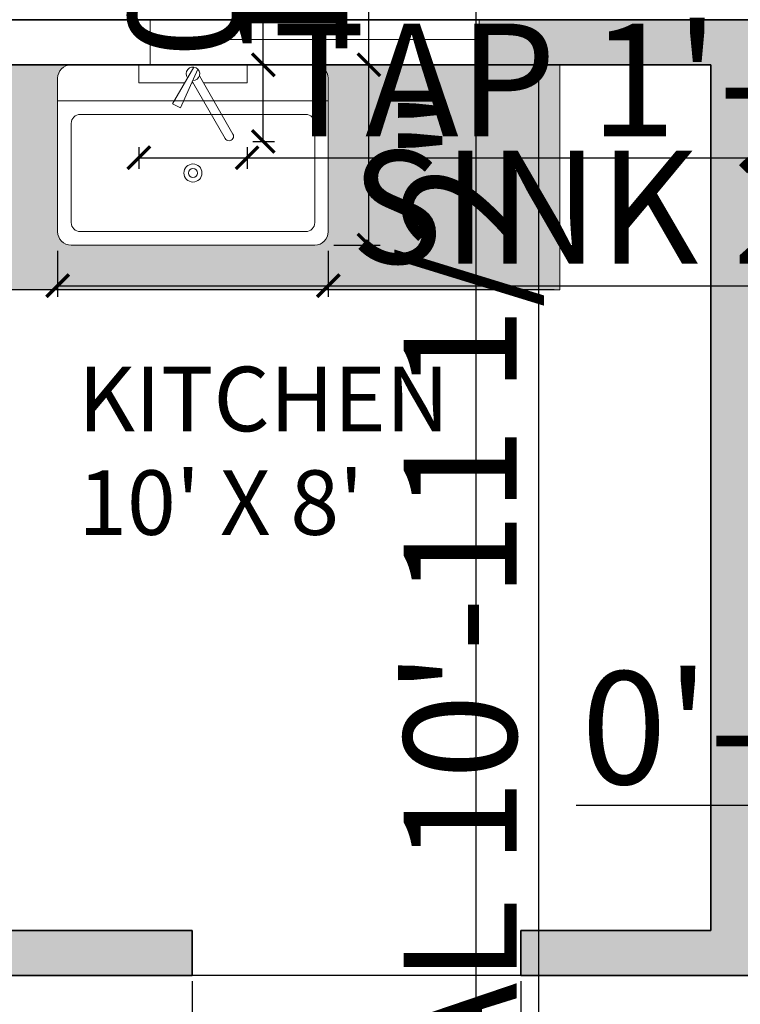
# Model space of a CAD drawing. Units: inches. Extents: x 1763 to 2368, y 1500 to 2097.
# Tile 8 of 24: x 1876 to 1956, y 1877 to 1986. Entities that reach past the tile are written whole.
import ezdxf

# ---------------------------------------------------------------- set-up
doc = ezdxf.new("R2010")
doc.units = ezdxf.units.IN
for name, color, linetype, lineweight in [('A-ANNO-DIMS', 2, 'Continuous', 18), ('A-AREA-IDEN', 7, 'Continuous', 18), ('A-FLOR-CASE', 8, 'Continuous', 18), ('A-FLOR-FIXT', 9, 'Continuous', 18), ('A-WALL', 7, 'Continuous', 35), ('A-WALL-PATT', 7, 'Continuous', 13), ('windows', 1, 'Continuous', 18)]:
    doc.layers.add(name, color=color, linetype=linetype, lineweight=lineweight)
doc.layers.add('A-FLOR-CASE-PATT', color=254, linetype='Continuous', lineweight=13, true_color=0xcecce6)
doc.styles.get("Standard").update_dxf_attribs({"font": 'arial.ttf'})
doc.dimstyles.new('ISO-25', dxfattribs={"dimtxt": 12.5, "dimasz": 2.5, "dimexe": 1.25, "dimexo": 0.625, "dimtad": 1, "dimdec": 0, "dimlunit": 4, "dimtxsty": 'Standard', "dimblk": 'ARCHTICK', "dimcen": 2.5, "dimclrd": 3, "dimclrt": 4, "dimadec": 0, "dimazin": 0, "dimtfac": 1, "dimtdec": 0, "dimtmove": 0, "dimatfit": 3, "dimfxl": 1, "dimarcsym": 0})

# ---------------------------------------------------------------- blocks, each defined once
blk = doc.blocks.new('Faucet - single handle top')
for p, q in [((0.08, -0.26), (-2.26, -4.34)), ((-1.37, -4.79), (0.55, -0.5)), ((-0.06, -1.9), (3.57, -8.18)), ((4.43, -7.68), (0.72, -1.24)), ((-2.26, -4.34), (-1.37, -4.79))]:
    blk.add_line(p, q)
for points in [[(-0.92, -2), (-6, -2), (-6, 0), (6, 0), (6, -2), (1.16, -2)], [(-0.01, -2), (-0.12, -2)]]:
    blk.add_lwpolyline(points)
for centre, radius, start, end in [((0, -1), 0.75, 269.2246, 216.2304), ((4, -7.93), 0.5, 210, 30)]:
    blk.add_arc(centre, radius, start, end)
blk = doc.blocks.new('Sink-single - 30 in top')
blk.add_line((-15, -3.999996), (15, -3.999996))
for points in [[(-13.5, 0), (13.5, 0)], [(-15, -18.499996), (-15, -1.5)], [(15, -1.5), (15, -18.499996)], [(-13.5, -17.499996), (-13.5, -6.499996)], [(-12.5, -5.499996), (12.5, -5.499996)], [(13.5, -6.499996), (13.5, -17.499996)], [(12.5, -18.499996), (-12.5, -18.499996)], [(13.5, -19.999996), (-13.5, -19.999996)]]:
    blk.add_lwpolyline(points)
for radius in [1, 0.5]:
    blk.add_circle((0, -11.999996), radius)
for centre, radius, start, end in [((-13.5, -1.5), 1.5, 90, 180), ((13.5, -1.5), 1.5, 0, 90), ((-12.5, -6.499996), 1, 90, 180), ((12.5, -6.499996), 1, 0, 90), ((-13.5, -18.499996), 1.5, 180, 270), ((-12.5, -17.499996), 1, 180, 270), ((12.5, -17.499996), 1, 270, 0), ((13.5, -18.499996), 1.5, 270, 0)]:
    blk.add_arc(centre, radius, start, end)
blk = doc.blocks.new('_ArchTick')
at = {"color": 0, "linetype": 'ByBlock', "const_width": 0.15}
blk.add_lwpolyline([(-0.5, -0.5), (0.5, 0.5)], dxfattribs=at)
blk = doc.blocks.new('*D25')
at = {"layer": 'A-ANNO-DIMS', "color": 3, "lineweight": -2, "transparency": 16777216}
for p, q in [((1934.01, 1792.31), (1934.01, 1981.61)), ((1934.01, 1660.94), (1934.01, 1792.31))]:
    blk.add_line(p, q, dxfattribs=at)
at = {"layer": 'A-ANNO-DIMS', "color": 0, "lineweight": -2, "transparency": 16777216}
for p, q in [((1953.09, 1792.31), (1932.76, 1792.31)), ((1953.09, 1660.94), (1932.76, 1660.94))]:
    blk.add_line(p, q, dxfattribs=at)
at = {"layer": 'Defpoints', "color": 0, "transparency": 16777216}
for p in [(1934.01, 1792.31), (1953.72, 1792.31), (1953.72, 1660.94)]:
    blk.add_point(p, dxfattribs=at)
at = {"layer": 'A-ANNO-DIMS', "color": 3, "lineweight": -2, "transparency": 16777216, "xscale": 2.5, "yscale": 2.5, "zscale": 2.5}
for p, rotation in [((1934.01, 1792.31), 90), ((1934.01, 1660.94), 270)]:
    blk.add_blockref('_ArchTick', p, dxfattribs=dict(at, rotation=rotation))
at = {"layer": 'A-ANNO-DIMS', "color": 4, "transparency": 16777216, "insert": (1926.92, 1888.21), "char_height": 12.5, "attachment_point": 5, "rotation": 90}
blk.add_mtext('SECTIONAL 10\'-11 1/2"', dxfattribs=at)
blk = doc.blocks.new('*D29')
at = {"layer": 'A-ANNO-DIMS', "color": 3, "lineweight": -2, "transparency": 16777216}
for p, q in [((1868.59, 1924.21), (1868.59, 2027.49)), ((1868.59, 1894.21), (1868.59, 1924.21))]:
    blk.add_line(p, q, dxfattribs=at)
at = {"layer": 'A-ANNO-DIMS', "color": 0, "lineweight": -2, "transparency": 16777216}
for p, q in [((1864.72, 1924.21), (1869.84, 1924.21)), ((1864.72, 1894.21), (1869.84, 1894.21))]:
    blk.add_line(p, q, dxfattribs=at)
at = {"layer": 'Defpoints', "color": 0, "transparency": 16777216}
for p in [(1864.09, 1924.21), (1868.59, 1924.21), (1864.09, 1894.21)]:
    blk.add_point(p, dxfattribs=at)
at = {"layer": 'A-ANNO-DIMS', "color": 3, "lineweight": -2, "transparency": 16777216, "xscale": 2.5, "yscale": 2.5, "zscale": 2.5}
for p, rotation in [((1868.59, 1924.21), 90), ((1868.59, 1894.21), 270)]:
    blk.add_blockref('_ArchTick', p, dxfattribs=dict(at, rotation=rotation))
at = {"layer": 'A-ANNO-DIMS', "color": 4, "transparency": 16777216, "insert": (1861.5, 1977.1), "char_height": 12.5, "attachment_point": 5, "rotation": 90}
blk.add_mtext('RANGE 2\'-6"', dxfattribs=at)
blk = doc.blocks.new('*D31')
at = {"layer": 'A-ANNO-DIMS', "color": 0, "lineweight": -2, "transparency": 16777216}
for p, q in [((1880.68, 1960.65), (1880.68, 1955.52)), ((1910.68, 1960.65), (1910.68, 1955.52))]:
    blk.add_line(p, q, dxfattribs=at)
at = {"layer": 'A-ANNO-DIMS', "color": 3, "lineweight": -2, "transparency": 16777216}
for p, q in [((1880.68, 1956.77), (1910.68, 1956.77)), ((1910.68, 1956.77), (1993.21, 1956.77))]:
    blk.add_line(p, q, dxfattribs=at)
at = {"layer": 'Defpoints', "color": 0, "transparency": 16777216}
for p in [(1880.68, 1961.27), (1910.68, 1961.27), (1910.68, 1956.77)]:
    blk.add_point(p, dxfattribs=at)
at = {"layer": 'A-ANNO-DIMS', "color": 3, "lineweight": -2, "transparency": 16777216, "xscale": 2.5, "yscale": 2.5, "zscale": 2.5, "rotation": 180}
blk.add_blockref('_ArchTick', (1880.68, 1956.77), dxfattribs=at)
at = {"layer": 'A-ANNO-DIMS', "color": 3, "lineweight": -2, "transparency": 16777216, "xscale": 2.5, "yscale": 2.5, "zscale": 2.5}
blk.add_blockref('_ArchTick', (1910.68, 1956.77), dxfattribs=at)
at = {"layer": 'A-ANNO-DIMS', "color": 4, "transparency": 16777216, "insert": (1953.2, 1963.86), "char_height": 12.5, "attachment_point": 5}
blk.add_mtext('SINK 2\'-6"', dxfattribs=at)
blk = doc.blocks.new('*D32')
at = {"layer": 'A-ANNO-DIMS', "color": 3, "lineweight": -2, "transparency": 16777216}
for p, q in [((1915.18, 1981.27), (1915.18, 2017.07)), ((1915.18, 1961.27), (1915.18, 1981.27))]:
    blk.add_line(p, q, dxfattribs=at)
at = {"layer": 'A-ANNO-DIMS', "color": 0, "lineweight": -2, "transparency": 16777216}
for p, q in [((1911.31, 1981.27), (1916.43, 1981.27)), ((1911.31, 1961.27), (1916.43, 1961.27))]:
    blk.add_line(p, q, dxfattribs=at)
at = {"layer": 'Defpoints', "color": 0, "transparency": 16777216}
for p in [(1910.68, 1981.27), (1915.18, 1981.27), (1910.68, 1961.27)]:
    blk.add_point(p, dxfattribs=at)
at = {"layer": 'A-ANNO-DIMS', "color": 3, "lineweight": -2, "transparency": 16777216, "xscale": 2.5, "yscale": 2.5, "zscale": 2.5}
for p, rotation in [((1915.18, 1981.27), 90), ((1915.18, 1961.27), 270)]:
    blk.add_blockref('_ArchTick', p, dxfattribs=dict(at, rotation=rotation))
at = {"layer": 'A-ANNO-DIMS', "color": 4, "transparency": 16777216, "insert": (1908.18, 2000.42), "char_height": 12.5, "attachment_point": 5, "rotation": 90}
blk.add_mtext('1\'-8"', dxfattribs=at)
blk = doc.blocks.new('*D35')
at = {"layer": 'A-ANNO-DIMS', "color": 0, "lineweight": -2, "transparency": 16777216}
for p, q in [((1889.68, 1972.15), (1889.68, 1969.72)), ((1901.68, 1972.15), (1901.68, 1969.72))]:
    blk.add_line(p, q, dxfattribs=at)
at = {"layer": 'A-ANNO-DIMS', "color": 3, "lineweight": -2, "transparency": 16777216}
for p, q in [((1889.68, 1970.97), (1901.68, 1970.97)), ((1901.68, 1970.97), (1977.79, 1970.97))]:
    blk.add_line(p, q, dxfattribs=at)
at = {"layer": 'Defpoints', "color": 0, "transparency": 16777216}
for p in [(1889.68, 1972.77), (1901.68, 1972.77), (1901.68, 1970.97)]:
    blk.add_point(p, dxfattribs=at)
at = {"layer": 'A-ANNO-DIMS', "color": 3, "lineweight": -2, "transparency": 16777216, "xscale": 2.5, "yscale": 2.5, "zscale": 2.5, "rotation": 180}
blk.add_blockref('_ArchTick', (1889.68, 1970.97), dxfattribs=at)
at = {"layer": 'A-ANNO-DIMS', "color": 3, "lineweight": -2, "transparency": 16777216, "xscale": 2.5, "yscale": 2.5, "zscale": 2.5}
blk.add_blockref('_ArchTick', (1901.68, 1970.97), dxfattribs=at)
at = {"layer": 'A-ANNO-DIMS', "color": 4, "transparency": 16777216, "insert": (1940.99, 1977.98), "char_height": 12.5, "attachment_point": 5}
blk.add_mtext('TAP 1\'-0"', dxfattribs=at)
blk = doc.blocks.new('*D36')
at = {"layer": 'A-ANNO-DIMS', "color": 3, "lineweight": -2, "transparency": 16777216}
for p, q in [((1903.48, 1981.27), (1903.48, 2047.38)), ((1903.48, 1972.77), (1903.48, 1981.27))]:
    blk.add_line(p, q, dxfattribs=at)
at = {"layer": 'A-ANNO-DIMS', "color": 0, "lineweight": -2, "transparency": 16777216}
for p, q in [((1902.31, 1981.27), (1904.73, 1981.27)), ((1902.31, 1972.77), (1904.73, 1972.77))]:
    blk.add_line(p, q, dxfattribs=at)
at = {"layer": 'Defpoints', "color": 0, "transparency": 16777216}
for p in [(1901.68, 1981.27), (1903.48, 1981.27), (1901.68, 1972.77)]:
    blk.add_point(p, dxfattribs=at)
at = {"layer": 'A-ANNO-DIMS', "color": 3, "lineweight": -2, "transparency": 16777216, "xscale": 2.5, "yscale": 2.5, "zscale": 2.5}
for p, rotation in [((1903.48, 1981.27), 90), ((1903.48, 1972.77), 270)]:
    blk.add_blockref('_ArchTick', p, dxfattribs=dict(at, rotation=rotation))
at = {"layer": 'A-ANNO-DIMS', "color": 4, "transparency": 16777216, "insert": (1896.4, 2015.58), "char_height": 12.5, "attachment_point": 5, "rotation": 90}
blk.add_mtext('0\'-8 1/2"', dxfattribs=at)
blk = doc.blocks.new('*D38')
at = {"layer": 'A-ANNO-DIMS', "color": 3, "lineweight": -2, "transparency": 16777216}
for p, q in [((2018.09, 1899.11), (1938.15, 1899.11)), ((2022.96, 1899.11), (2018.09, 1899.11))]:
    blk.add_line(p, q, dxfattribs=at)
at = {"layer": 'A-ANNO-DIMS', "color": 0, "lineweight": -2, "transparency": 16777216}
for p, q in [((2018.09, 1899.52), (2018.09, 1897.86)), ((2022.96, 1899.52), (2022.96, 1897.86))]:
    blk.add_line(p, q, dxfattribs=at)
at = {"layer": 'Defpoints', "color": 0, "transparency": 16777216}
for p in [(2018.09, 1900.14), (2022.96, 1900.14), (2018.09, 1899.11)]:
    blk.add_point(p, dxfattribs=at)
at = {"layer": 'A-ANNO-DIMS', "color": 3, "lineweight": -2, "transparency": 16777216, "xscale": 2.5, "yscale": 2.5, "zscale": 2.5, "rotation": 180}
blk.add_blockref('_ArchTick', (2018.09, 1899.11), dxfattribs=at)
at = {"layer": 'A-ANNO-DIMS', "color": 3, "lineweight": -2, "transparency": 16777216, "xscale": 2.5, "yscale": 2.5, "zscale": 2.5}
blk.add_blockref('_ArchTick', (2022.96, 1899.11), dxfattribs=at)
at = {"layer": 'A-ANNO-DIMS', "color": 4, "transparency": 16777216, "insert": (1976.87, 1906.12), "char_height": 12.5, "attachment_point": 5}
blk.add_mtext('0\'-5" TYP.', dxfattribs=at)
blk = doc.blocks.new('*D58')
at = {"layer": 'A-ANNO-DIMS', "color": 0, "lineweight": -2, "transparency": 16777216}
for p, q in [((1871.68, 1635.9), (1871.68, 2072.02)), ((1927.07, 1635.9), (1927.07, 2072.02))]:
    blk.add_line(p, q, dxfattribs=at)
at = {"layer": 'A-ANNO-DIMS', "color": 3, "lineweight": -2, "transparency": 16777216}
for p, q in [((1871.68, 2070.77), (1927.07, 2070.77)), ((1927.07, 2070.77), (1993.68, 2070.77))]:
    blk.add_line(p, q, dxfattribs=at)
at = {"layer": 'Defpoints', "color": 0, "transparency": 16777216}
for p in [(1927.07, 2070.77), (1871.68, 1635.27), (1927.07, 1635.27)]:
    blk.add_point(p, dxfattribs=at)
at = {"layer": 'A-ANNO-DIMS', "color": 3, "lineweight": -2, "transparency": 16777216, "xscale": 2.5, "yscale": 2.5, "zscale": 2.5, "rotation": 180}
blk.add_blockref('_ArchTick', (1871.68, 2070.77), dxfattribs=at)
at = {"layer": 'A-ANNO-DIMS', "color": 3, "lineweight": -2, "transparency": 16777216, "xscale": 2.5, "yscale": 2.5, "zscale": 2.5}
blk.add_blockref('_ArchTick', (1927.07, 2070.77), dxfattribs=at)
at = {"layer": 'A-ANNO-DIMS', "color": 4, "transparency": 16777216, "insert": (1961.63, 2077.86), "char_height": 12.5, "attachment_point": 5}
blk.add_mtext('4\'-7 1/2"', dxfattribs=at)
blk = doc.blocks.new('*D68')
at = {"layer": 'A-ANNO-DIMS', "color": 0, "lineweight": -2, "transparency": 16777216}
for p, q in [((1895.59, 1879.65), (1895.59, 1509.91)), ((1932.01, 1879.65), (1932.01, 1509.91))]:
    blk.add_line(p, q, dxfattribs=at)
at = {"layer": 'A-ANNO-DIMS', "color": 3, "lineweight": -2, "transparency": 16777216}
for p, q in [((1895.59, 1511.16), (1932.01, 1511.16)), ((1932.01, 1511.16), (1998.11, 1511.16))]:
    blk.add_line(p, q, dxfattribs=at)
at = {"layer": 'Defpoints', "color": 0, "transparency": 16777216}
for p in [(1895.59, 1880.27), (1932.01, 1880.27), (1932.01, 1511.16)]:
    blk.add_point(p, dxfattribs=at)
at = {"layer": 'A-ANNO-DIMS', "color": 3, "lineweight": -2, "transparency": 16777216, "xscale": 2.5, "yscale": 2.5, "zscale": 2.5, "rotation": 180}
blk.add_blockref('_ArchTick', (1895.59, 1511.16), dxfattribs=at)
at = {"layer": 'A-ANNO-DIMS', "color": 3, "lineweight": -2, "transparency": 16777216, "xscale": 2.5, "yscale": 2.5, "zscale": 2.5}
blk.add_blockref('_ArchTick', (1932.01, 1511.16), dxfattribs=at)
at = {"layer": 'A-ANNO-DIMS', "color": 4, "transparency": 16777216, "insert": (1966.31, 1518.25), "char_height": 12.5, "attachment_point": 5}
blk.add_mtext('3\'-0 1/2"', dxfattribs=at)
blk = doc.blocks.new('*D69')
at = {"layer": 'A-ANNO-DIMS', "color": 0, "lineweight": -2, "transparency": 16777216}
for p, q in [((1838.09, 1879.65), (1838.09, 1509.91)), ((1895.59, 1879.65), (1895.59, 1509.91))]:
    blk.add_line(p, q, dxfattribs=at)
at = {"layer": 'A-ANNO-DIMS', "color": 3, "lineweight": -2, "transparency": 16777216}
for p, q in [((1838.09, 1511.16), (1895.59, 1511.16)), ((1895.59, 1511.16), (1962.2, 1511.16))]:
    blk.add_line(p, q, dxfattribs=at)
at = {"layer": 'Defpoints', "color": 0, "transparency": 16777216}
for p in [(1838.09, 1880.27), (1895.59, 1880.27), (1895.59, 1511.16)]:
    blk.add_point(p, dxfattribs=at)
at = {"layer": 'A-ANNO-DIMS', "color": 3, "lineweight": -2, "transparency": 16777216, "xscale": 2.5, "yscale": 2.5, "zscale": 2.5, "rotation": 180}
blk.add_blockref('_ArchTick', (1838.09, 1511.16), dxfattribs=at)
at = {"layer": 'A-ANNO-DIMS', "color": 3, "lineweight": -2, "transparency": 16777216, "xscale": 2.5, "yscale": 2.5, "zscale": 2.5}
blk.add_blockref('_ArchTick', (1895.59, 1511.16), dxfattribs=at)
at = {"layer": 'A-ANNO-DIMS', "color": 4, "transparency": 16777216, "insert": (1930.15, 1518.24), "char_height": 12.5, "attachment_point": 5}
blk.add_mtext('4\'-9 1/2"', dxfattribs=at)
blk = doc.blocks.new('*D81')
at = {"layer": 'A-ANNO-DIMS', "color": 3, "lineweight": -2, "transparency": 16777216}
for p, q in [((1788.85, 1866.87), (1788.85, 1912.38)), ((1788.85, 1843.77), (1788.85, 1866.87))]:
    blk.add_line(p, q, dxfattribs=at)
at = {"layer": 'A-ANNO-DIMS', "color": 0, "lineweight": -2, "transparency": 16777216}
for p, q in [((2077.47, 1866.87), (1787.6, 1866.87)), ((2077.47, 1843.77), (1787.6, 1843.77))]:
    blk.add_line(p, q, dxfattribs=at)
at = {"layer": 'Defpoints', "color": 0, "transparency": 16777216}
for p in [(1788.85, 1866.87), (2078.09, 1866.87), (2078.09, 1843.77)]:
    blk.add_point(p, dxfattribs=at)
at = {"layer": 'A-ANNO-DIMS', "color": 3, "lineweight": -2, "transparency": 16777216, "xscale": 2.5, "yscale": 2.5, "zscale": 2.5}
for p, rotation in [((1788.85, 1866.87), 90), ((1788.85, 1843.77), 270)]:
    blk.add_blockref('_ArchTick', p, dxfattribs=dict(at, rotation=rotation))
at = {"layer": 'A-ANNO-DIMS', "color": 4, "transparency": 16777216, "insert": (1781.95, 1890.87), "char_height": 12.5, "attachment_point": 5, "rotation": 90}
blk.add_mtext('1\'-11"', dxfattribs=at)
blk = doc.blocks.new('*D82')
at = {"layer": 'A-ANNO-DIMS', "color": 3, "lineweight": -2, "transparency": 16777216}
for p, q in [((1788.85, 1843.77), (1788.85, 1909.87)), ((1788.85, 1837.27), (1788.85, 1843.77))]:
    blk.add_line(p, q, dxfattribs=at)
at = {"layer": 'A-ANNO-DIMS', "color": 0, "lineweight": -2, "transparency": 16777216}
for p, q in [((2077.47, 1843.77), (1787.6, 1843.77)), ((2077.47, 1837.27), (1787.6, 1837.27))]:
    blk.add_line(p, q, dxfattribs=at)
at = {"layer": 'Defpoints', "color": 0, "transparency": 16777216}
for p in [(1788.85, 1843.77), (2078.09, 1843.77), (2078.09, 1837.27)]:
    blk.add_point(p, dxfattribs=at)
at = {"layer": 'A-ANNO-DIMS', "color": 3, "lineweight": -2, "transparency": 16777216, "xscale": 2.5, "yscale": 2.5, "zscale": 2.5}
for p, rotation in [((1788.85, 1843.77), 90), ((1788.85, 1837.27), 270)]:
    blk.add_blockref('_ArchTick', p, dxfattribs=dict(at, rotation=rotation))
at = {"layer": 'A-ANNO-DIMS', "color": 4, "transparency": 16777216, "insert": (1781.77, 1878.07), "char_height": 12.5, "attachment_point": 5, "rotation": 90}
blk.add_mtext('0\'-6 1/2"', dxfattribs=at)
blk = doc.blocks.new('*D85')
at = {"layer": 'A-ANNO-DIMS', "color": 0, "lineweight": -2, "transparency": 16777216}
for p, q in [((1957.47, 1986.27), (1787.6, 1986.27)), ((1958.51, 1880.27), (1787.6, 1880.27))]:
    blk.add_line(p, q, dxfattribs=at)
at = {"layer": 'A-ANNO-DIMS', "color": 3, "lineweight": -2, "transparency": 16777216}
blk.add_line((1788.85, 1986.27), (1788.85, 1880.27), dxfattribs=at)
at = {"layer": 'Defpoints', "color": 0, "transparency": 16777216}
for p in [(1958.09, 1986.27), (1788.85, 1880.27), (1959.13, 1880.27)]:
    blk.add_point(p, dxfattribs=at)
at = {"layer": 'A-ANNO-DIMS', "color": 3, "lineweight": -2, "transparency": 16777216, "xscale": 2.5, "yscale": 2.5, "zscale": 2.5}
for p, rotation in [((1788.85, 1986.27), 90), ((1788.85, 1880.27), 270)]:
    blk.add_blockref('_ArchTick', p, dxfattribs=dict(at, rotation=rotation))
at = {"layer": 'A-ANNO-DIMS', "color": 4, "transparency": 16777216, "insert": (1781.85, 1933.27), "char_height": 12.5, "attachment_point": 5, "rotation": 90}
blk.add_mtext('8\'-10"', dxfattribs=at)
blk = doc.blocks.new('*D90')
at = {"layer": 'A-ANNO-DIMS', "color": 0, "lineweight": -2, "transparency": 16777216}
for p, q in [((1838.09, 1980.65), (1838.09, 1509.91)), ((1866.04, 1955.7), (1866.04, 1509.91))]:
    blk.add_line(p, q, dxfattribs=at)
at = {"layer": 'A-ANNO-DIMS', "color": 3, "lineweight": -2, "transparency": 16777216}
for p, q in [((1838.09, 1511.16), (1866.04, 1511.16)), ((1866.04, 1511.16), (1903.23, 1511.16))]:
    blk.add_line(p, q, dxfattribs=at)
at = {"layer": 'Defpoints', "color": 0, "transparency": 16777216}
for p in [(1838.09, 1981.27), (1866.04, 1956.32), (1866.04, 1511.16)]:
    blk.add_point(p, dxfattribs=at)
at = {"layer": 'A-ANNO-DIMS', "color": 3, "lineweight": -2, "transparency": 16777216, "xscale": 2.5, "yscale": 2.5, "zscale": 2.5, "rotation": 180}
blk.add_blockref('_ArchTick', (1838.09, 1511.16), dxfattribs=at)
at = {"layer": 'A-ANNO-DIMS', "color": 3, "lineweight": -2, "transparency": 16777216, "xscale": 2.5, "yscale": 2.5, "zscale": 2.5}
blk.add_blockref('_ArchTick', (1866.04, 1511.16), dxfattribs=at)
at = {"layer": 'A-ANNO-DIMS', "color": 4, "transparency": 16777216, "insert": (1885.88, 1518.06), "char_height": 12.5, "attachment_point": 5}
blk.add_mtext('2\'-4"', dxfattribs=at)
blk = doc.blocks.new('*D91')
at = {"layer": 'A-ANNO-DIMS', "color": 0, "lineweight": -2, "transparency": 16777216}
for p, q in [((1935.72, 1981.27), (1787.6, 1981.27)), ((1935.72, 1956.32), (1787.6, 1956.32))]:
    blk.add_line(p, q, dxfattribs=at)
at = {"layer": 'A-ANNO-DIMS', "color": 3, "lineweight": -2, "transparency": 16777216}
for p, q in [((1788.85, 1981.27), (1788.85, 1956.32)), ((1788.85, 1956.32), (1788.85, 1919.13))]:
    blk.add_line(p, q, dxfattribs=at)
at = {"layer": 'Defpoints', "color": 0, "transparency": 16777216}
for p in [(1936.34, 1981.27), (1788.85, 1956.32), (1936.34, 1956.32)]:
    blk.add_point(p, dxfattribs=at)
at = {"layer": 'A-ANNO-DIMS', "color": 3, "lineweight": -2, "transparency": 16777216, "xscale": 2.5, "yscale": 2.5, "zscale": 2.5}
for p, rotation in [((1788.85, 1981.27), 90), ((1788.85, 1956.32), 270)]:
    blk.add_blockref('_ArchTick', p, dxfattribs=dict(at, rotation=rotation))
at = {"layer": 'A-ANNO-DIMS', "color": 4, "transparency": 16777216, "insert": (1781.95, 1936.48), "char_height": 12.5, "attachment_point": 5, "rotation": 90}
blk.add_mtext('2\'-1"', dxfattribs=at)

msp = doc.modelspace()

# ---------------------------------------------------------------- hatches: boundary and pattern name
at = {"layer": 'A-FLOR-CASE-PATT'}
h = msp.add_hatch(color=256, dxfattribs=at)
h.dxf.hatch_style = 1
h.paths.add_polyline_path([(1866.04, 1956.32), (1936.34, 1956.32), (1936.34, 1981.27), (1909.18, 1981.27, -0.414214), (1910.68, 1979.77), (1910.68, 1962.77, -0.414214), (1909.18, 1961.27), (1882.18, 1961.27, -0.414214), (1880.68, 1962.77), (1880.68, 1979.77, -0.414214), (1882.18, 1981.27), (1868.32, 1981.27), (1845.22, 1981.27), (1838.09, 1981.27), (1838.09, 1924.21), (1862.09, 1924.21), (1862.09, 1918.21), (1863.09, 1918.21), (1863.09, 1922.21), (1864.09, 1922.21), (1864.09, 1896.21), (1863.09, 1896.21), (1863.09, 1900.21), (1862.09, 1900.21), (1862.09, 1894.21), (1838.09, 1894.21), (1838.09, 1885.27), (1866.04, 1885.27)])
at = {"layer": 'A-WALL-PATT'}
h = msp.add_hatch(color=256, dxfattribs=at)
h.dxf.hatch_style = 1
h.paths.add_polyline_path([(1838.09, 2034.27), (1838.09, 2043.27), (1829.09, 2043.27), (1829.09, 1953.39), (1838.09, 1953.39)])
h.paths.add_polyline_path([(1838.09, 1913.1), (1829.09, 1913.1), (1829.09, 1862.2), (1838.09, 1862.2)])
h.paths.add_polyline_path([(1838.09, 1825.59), (1829.09, 1825.59), (1829.09, 1738.64), (1838.09, 1738.64)])
h.paths.add_polyline_path([(1895.59, 1885.27), (1838.09, 1885.27), (1838.09, 1880.27), (1895.59, 1880.27)])
h.paths.add_polyline_path([(1857.39, 1784.27), (1838.09, 1784.27), (1838.09, 1779.27), (1857.39, 1779.27)])
h.paths.add_polyline_path([(1958.09, 1981.27), (1971.46, 1981.27), (1971.46, 1986.27), (1968.57, 1986.27), (1958.09, 1986.27), (1953.09, 1986.27), (1927.39, 1986.27), (1927.39, 1981.27), (1953.09, 1981.27), (1953.09, 1885.27), (1932.01, 1885.27), (1932.01, 1880.27), (1959.13, 1880.27), (1959.13, 1883.74), (1959.13, 1885.27), (1958.09, 1885.27)])
h.paths.add_polyline_path([(2018.09, 1981.27), (2031.02, 1981.27), (2031.02, 1986.27), (2018.09, 1986.27), (2013.09, 1986.27), (2001.23, 1986.27), (2001.23, 1981.27), (2013.09, 1981.27), (2013.09, 1885.27), (1982.18, 1885.27, -0.016629), (1982.23, 1883.74), (1982.23, 1880.27), (2049.69, 1880.27), (2049.69, 1883.74, -0.016629), (2049.74, 1885.27), (2018.09, 1885.27)])
h.paths.add_polyline_path([(2083.09, 1981.27), (2120.61, 1981.27), (2120.61, 1986.27), (2083.09, 1986.27), (2078.09, 1986.27), (2063.14, 1986.27), (2063.14, 1981.27), (2078.09, 1981.27), (2078.09, 1885.27), (2072.78, 1885.27), (2072.78, 1883.74), (2072.78, 1880.27), (2078.09, 1880.27), (2078.09, 1866.87), (2081.56, 1866.87, -0.016629), (2083.09, 1866.82)])
h.paths.add_polyline_path([(1871.68, 1635.27), (1838.09, 1635.27), (1838.09, 1626.27), (1871.68, 1626.27)], flags=17)
h.paths.add_polyline_path([(2100.58, 1688.27), (2060.09, 1688.27), (2060.09, 1679.27), (2100.58, 1679.27)], flags=17)
h.paths.add_polyline_path([(2180.09, 1688.27), (2148.74, 1688.27), (2148.74, 1679.27), (2180.09, 1679.27)], flags=17)
h.paths.add_polyline_path([(2189.09, 1746.22), (2180.09, 1746.22), (2180.09, 1743.42), (2180.12, 1743.42), (2180.12, 1726.72), (2180.09, 1572.27), (2034.91, 1572.27), (2034.91, 1565.6), (2034.91, 1563.27), (2189.09, 1563.27)])
h.paths.add_polyline_path([(2060.09, 1802.35, -0.016629), (2058.56, 1802.3), (2055.09, 1802.3), (2055.09, 1635.27), (2042.48, 1635.27), (2042.48, 1629.74), (2042.48, 1626.27), (2055.09, 1626.27), (2055.09, 1599.27), (2040.27, 1599.27), (2040.27, 1590.27), (2060.09, 1590.27)])
h.paths.add_polyline_path([(2019.39, 1629.74, -0.060569), (2020.06, 1635.27), (1995.09, 1635.27), (1990.09, 1635.27), (1927.07, 1635.27), (1927.07, 1626.27), (1990.09, 1626.27), (1990.09, 1590.27), (1995.09, 1590.27), (2005.2, 1590.27), (2005.2, 1599.27), (1995.09, 1599.27), (1995.09, 1626.27), (2019.39, 1626.27)])
edge = h.paths.add_edge_path()
edge.add_line((2180.09, 1837.27), (2167.2, 1837.27))
edge.add_spline(control_points=[(2167.2, 1837.27), (2167.19, 1837.27), (2167.18, 1837.27), (2167.18, 1837.27)], knot_values=[168.955493, 168.955493, 168.955493, 168.955493, 169.065871, 169.065871, 169.065871, 169.065871], degree=3, periodic=0)
edge.add_spline(control_points=[(2167.18, 1837.27), (2166.56, 1837.38), (2166.33, 1846.16), (2165.71, 1846.24)], knot_values=[159.864705, 159.864705, 159.864705, 159.864705, 168.955493, 168.955493, 168.955493, 168.955493], degree=3, periodic=0)
edge.add_line((2167.12, 1837.27), (2163.16, 1837.27))
edge.add_spline(control_points=[(2163.16, 1837.27), (2163.16, 1837.27), (2163.16, 1837.27), (2163.15, 1837.27)], knot_values=[150.537172, 150.537172, 150.537172, 150.537172, 150.553797, 150.553797, 150.553797, 150.553797], degree=3, periodic=0)
edge.add_spline(control_points=[(2163.15, 1837.27), (2162.29, 1837.29), (2161.59, 1846.23), (2160.88, 1846.24)], knot_values=[141.293426, 141.293426, 141.293426, 141.293426, 150.537172, 150.537172, 150.537172, 150.537172], degree=3, periodic=0)
edge.add_line((2163.08, 1837.27), (2158.7, 1837.27))
edge.add_spline(control_points=[(2158.7, 1837.27), (2158.7, 1837.27), (2158.7, 1837.27), (2158.7, 1837.27)], knot_values=[132.033544, 132.033544, 132.033544, 132.033544, 132.049151, 132.049151, 132.049151, 132.049151], degree=3, periodic=0)
edge.add_spline(control_points=[(2158.7, 1837.27), (2157.97, 1837.29), (2157.26, 1846.23), (2156.39, 1846.24)], knot_values=[122.786021, 122.786021, 122.786021, 122.786021, 132.033544, 132.033544, 132.033544, 132.033544], degree=3, periodic=0)
edge.add_line((2158.63, 1837.27), (2153.84, 1837.27))
edge.add_spline(control_points=[(2153.84, 1837.27), (2153.83, 1837.27), (2153.82, 1837.27), (2153.82, 1837.27)], knot_values=[113.451585, 113.451585, 113.451585, 113.451585, 113.562103, 113.562103, 113.562103, 113.562103], degree=3, periodic=0)
edge.add_spline(control_points=[(2153.82, 1837.27), (2153.17, 1837.38), (2152.88, 1846.19), (2152.4, 1846.24)], knot_values=[0, 0, 0, 0, 9.081854, 9.081854, 9.081854, 9.081854], degree=3, periodic=0)
edge.add_line((2153.76, 1837.27), (2150.39, 1837.27))
edge.add_spline(control_points=[(2150.39, 1837.27), (2150.38, 1837.27), (2150.37, 1837.27), (2150.36, 1837.27)], knot_values=[95.069382, 95.069382, 95.069382, 95.069382, 95.17519, 95.17519, 95.17519, 95.17519], degree=3, periodic=0)
edge.add_spline(control_points=[(2150.36, 1837.27), (2149.49, 1837.37), (2148.42, 1846.19), (2147.59, 1846.24)], knot_values=[85.824599, 85.824599, 85.824599, 85.824599, 95.069382, 95.069382, 95.069382, 95.069382], degree=3, periodic=0)
edge.add_line((2150.29, 1837.27), (2145.43, 1837.27))
edge.add_spline(control_points=[(2145.43, 1837.27), (2145.43, 1837.27), (2145.42, 1837.27), (2145.42, 1837.27)], knot_values=[76.505559, 76.505559, 76.505559, 76.505559, 76.547811, 76.547811, 76.547811, 76.547811], degree=3, periodic=0)
edge.add_spline(control_points=[(2145.42, 1837.27), (2144.68, 1837.31), (2143.8, 1846.19), (2142.95, 1846.24)], knot_values=[67.23945, 67.23945, 67.23945, 67.23945, 76.505559, 76.505559, 76.505559, 76.505559], degree=3, periodic=0)
edge.add_line((2145.35, 1837.27), (2134.57, 1837.27))
edge.add_spline(control_points=[(2134.57, 1837.27), (2134.57, 1837.27), (2134.56, 1837.27), (2134.56, 1837.27)], knot_values=[39.001463, 39.001463, 39.001463, 39.001463, 39.045107, 39.045107, 39.045107, 39.045107], degree=3, periodic=0)
edge.add_spline(control_points=[(2134.56, 1837.27), (2133.87, 1837.31), (2133.4, 1845.85), (2132.33, 1846.24)], knot_values=[29.79778, 29.79778, 29.79778, 29.79778, 39.001463, 39.001463, 39.001463, 39.001463], degree=3, periodic=0)
edge.add_line((2134.5, 1837.27), (2128.08, 1837.27))
edge.add_spline(control_points=[(2128.08, 1837.27), (2128.03, 1837.26), (2127.98, 1837.26), (2127.93, 1837.27)], knot_values=[19.482067, 19.482067, 19.482067, 19.482067, 19.869396, 19.869396, 19.869396, 19.869396], degree=3, periodic=0)
edge.add_spline(control_points=[(2125.01, 1846.24), (2126.16, 1844.66), (2126.82, 1837.57), (2127.93, 1837.27)], knot_values=[10.389805, 10.389805, 10.389805, 10.389805, 19.482067, 19.482067, 19.482067, 19.482067], degree=3, periodic=0)
edge.add_line((2127.93, 1837.27), (2083.09, 1837.27))
edge.add_line((2083.09, 1837.27), (2083.09, 1843.77))
edge.add_line((2083.09, 1843.77), (2081.56, 1843.77))
edge.add_line((2081.56, 1843.77), (2078.09, 1843.77))
edge.add_line((2078.09, 1843.77), (2078.09, 1837.27))
edge.add_line((2078.09, 1837.27), (2055.09, 1837.27))
edge.add_line((2055.09, 1837.27), (2055.09, 1825.4))
edge.add_line((2055.09, 1825.4), (2058.56, 1825.4))
edge.add_line((2058.56, 1825.4), (2060.09, 1825.4))
edge.add_line((2060.09, 1825.4), (2060.09, 1832.27))
edge.add_line((2060.09, 1832.27), (2122.44, 1832.27))
edge.add_spline(control_points=[(2122.44, 1832.27), (2122.73, 1832.58), (2123.01, 1832.62), (2123.28, 1832.27)], knot_values=[5.972033, 5.972033, 5.972033, 5.972033, 8.057258, 8.057258, 8.057258, 8.057258], degree=3, periodic=0)
edge.add_line((2123.28, 1832.27), (2137.95, 1832.27))
edge.add_spline(control_points=[(2137.95, 1832.27), (2137.96, 1832.27), (2137.97, 1832.27), (2137.98, 1832.27)], knot_values=[53.926862, 53.926862, 53.926862, 53.926862, 54.030075, 54.030075, 54.030075, 54.030075], degree=3, periodic=0)
edge.add_spline(control_points=[(2139.72, 1825.02), (2139.28, 1825.06), (2138.67, 1832.18), (2137.98, 1832.27)], knot_values=[54.030075, 54.030075, 54.030075, 54.030075, 61.445194, 61.445194, 61.445194, 61.445194], degree=3, periodic=0)
edge.add_line((2138.05, 1832.27), (2140.96, 1832.27))
edge.add_spline(control_points=[(2140.96, 1832.27), (2140.97, 1832.27), (2140.98, 1832.27), (2140.99, 1832.27)], knot_values=[68.854182, 68.854182, 68.854182, 68.854182, 68.971237, 68.971237, 68.971237, 68.971237], degree=3, periodic=0)
edge.add_spline(control_points=[(2143.19, 1825.02), (2142.44, 1825.07), (2141.56, 1832.16), (2140.99, 1832.27)], knot_values=[68.971237, 68.971237, 68.971237, 68.971237, 76.444911, 76.444911, 76.444911, 76.444911], degree=3, periodic=0)
edge.add_line((2141.04, 1832.27), (2145.43, 1832.27))
edge.add_spline(control_points=[(2145.43, 1832.27), (2145.44, 1832.27), (2145.45, 1832.27), (2145.46, 1832.27)], knot_values=[84.039047, 84.039047, 84.039047, 84.039047, 84.124041, 84.124041, 84.124041, 84.124041], degree=3, periodic=0)
edge.add_spline(control_points=[(2148.11, 1825.02), (2147.34, 1825.02), (2146.3, 1832.19), (2145.46, 1832.27)], knot_values=[84.124041, 84.124041, 84.124041, 84.124041, 91.773891, 91.773891, 91.773891, 91.773891], degree=3, periodic=0)
edge.add_line((2145.54, 1832.27), (2150.39, 1832.27))
edge.add_spline(control_points=[(2150.39, 1832.27), (2150.42, 1832.28), (2150.45, 1832.28), (2150.47, 1832.27)], knot_values=[99.381577, 99.381577, 99.381577, 99.381577, 99.573457, 99.573457, 99.573457, 99.573457], degree=3, periodic=0)
edge.add_spline(control_points=[(2153.97, 1825.02), (2153.09, 1825.28), (2151.53, 1832.1), (2150.47, 1832.27)], knot_values=[99.573457, 99.573457, 99.573457, 99.573457, 107.218357, 107.218357, 107.218357, 107.218357], degree=3, periodic=0)
edge.add_line((2150.57, 1832.27), (2155.6, 1832.27))
edge.add_spline(control_points=[(2155.6, 1832.27), (2155.6, 1832.27), (2155.61, 1832.27), (2155.62, 1832.27)], knot_values=[114.933058, 114.933058, 114.933058, 114.933058, 115.013624, 115.013624, 115.013624, 115.013624], degree=3, periodic=0)
edge.add_spline(control_points=[(2158.28, 1825.02), (2157.4, 1825.07), (2156.25, 1832.2), (2155.62, 1832.27)], knot_values=[115.013624, 115.013624, 115.013624, 115.013624, 122.616269, 122.616269, 122.616269, 122.616269], degree=3, periodic=0)
edge.add_line((2155.68, 1832.27), (2165.19, 1832.27))
edge.add_spline(control_points=[(2165.19, 1832.27), (2165.2, 1832.27), (2165.2, 1832.27), (2165.2, 1832.27)], knot_values=[145.488477, 145.488477, 145.488477, 145.488477, 145.516379, 145.516379, 145.516379, 145.516379], degree=3, periodic=0)
edge.add_spline(control_points=[(2167.45, 1825.02), (2166.96, 1825.02), (2166.06, 1832.25), (2165.2, 1832.27)], knot_values=[145.516379, 145.516379, 145.516379, 145.516379, 153.105469, 153.105469, 153.105469, 153.105469], degree=3, periodic=0)
edge.add_line((2165.29, 1832.27), (2168.93, 1832.27))
edge.add_spline(control_points=[(2168.93, 1832.27), (2168.98, 1832.29), (2169.04, 1832.29), (2169.1, 1832.27)], knot_values=[160.517439, 160.517439, 160.517439, 160.517439, 160.939723, 160.939723, 160.939723, 160.939723], degree=3, periodic=0)
edge.add_spline(control_points=[(2171.09, 1828.64), (2170.35, 1830.37), (2169.62, 1832.09), (2169.1, 1832.27)], knot_values=[160.939723, 160.939723, 160.939723, 160.939723, 164.738835, 164.738835, 164.738835, 164.738835], degree=3, periodic=0)
edge.add_line((2169.1, 1832.27), (2180.09, 1832.27))
edge.add_line((2180.09, 1832.27), (2180.09, 1837.27))
h.paths.add_polyline_path([(2189.09, 1885.52), (2180.09, 1885.52), (2180.09, 1813.32), (2180.12, 1813.32), (2180.12, 1796.62), (2180.12, 1795.26), (2189.09, 1795.26)])
h.paths.add_polyline_path([(2180.09, 1986.27), (2166.28, 1986.27), (2166.28, 1981.27), (2180.09, 1981.27)])
h.paths.add_polyline_path([(2189.09, 2043.27), (2180.09, 2043.27), (2180.09, 2034.27), (2180.09, 1934.11), (2189.09, 1934.11)])
h.paths.add_polyline_path([(1838.09, 1681.59), (1829.09, 1681.59), (1829.09, 1563.27), (2003.86, 1563.27), (2003.86, 1565.6), (2003.86, 1572.27), (1838.09, 1572.27)])

# ---------------------------------------------------------------- linework, layer by layer
at = {"layer": 'A-FLOR-CASE'}
for p, q in [((1936.34, 1981.27), (1936.34, 1956.32)), ((1936.34, 1956.32), (1866.04, 1956.32))]:
    msp.add_line(p, q, dxfattribs=at)
at = {"layer": 'A-WALL'}
for p, q in [((1868.27, 1986.27), (1953.09, 1986.27)), ((1953.09, 1986.27), (1958.09, 1986.27)), ((1868.32, 1981.27), (1953.09, 1981.27)), ((1953.09, 1885.27), (1953.09, 1981.27)), ((1838.09, 1885.27), (1895.59, 1885.27)), ((1895.59, 1885.27), (1895.59, 1880.27)), ((1932.01, 1885.27), (1932.01, 1880.27)), ((1932.01, 1885.27), (1953.09, 1885.27)), ((1838.09, 1880.27), (1895.59, 1880.27)), ((1932.01, 1880.27), (1959.13, 1880.27))]:
    msp.add_line(p, q, dxfattribs=at)
at = {"layer": 'windows'}
for p, q in [((1890.93, 1986.27), (1890.93, 1981.27)), ((1927.39, 1986.27), (1890.93, 1986.27)), ((1927.39, 1981.27), (1927.39, 1986.27)), ((1927.39, 1984.07), (1890.93, 1984.07)), ((1890.93, 1981.27), (1927.39, 1981.27)), ((1927.39, 1981.27), (1890.93, 1981.27)), ((1927.39, 1981.27), (1890.93, 1981.27))]:
    msp.add_line(p, q, dxfattribs=at)

# ---------------------------------------------------------------- block references
at = {"layer": 'A-FLOR-FIXT'}
for name in ['Sink-single - 30 in top', 'Faucet - single handle top']:
    msp.add_blockref(name, (1895.68, 1981.27), dxfattribs=at)

# ---------------------------------------------------------------- texts
at = {"layer": 'A-AREA-IDEN'}
for s, p in [('KITCHEN', (1882.95, 1940.63)), ("10' X 8'", (1882.95, 1929.14))]:
    msp.add_text(s, height=7.155, dxfattribs=at).set_placement(p)

# ---------------------------------------------------------------- dimensions: what is measured, and where the dimension line sits
at = {"layer": 'A-ANNO-DIMS'}
for base, p1, p2, picture, middle in [((1927.07, 2070.77), (1871.68, 1635.27), (1927.07, 1635.27), '*D58', (1961.63, 2077.86)), ((1866.0388, 1511.1561), (1838.0918, 1981.2727), (1866.0388, 1956.3234), '*D90', (1885.8845, 1518.0567)), ((1895.59, 1511.16), (1838.09, 1880.27), (1895.59, 1880.27), '*D69', (1930.15, 1518.24)), ((1932.01, 1511.16), (1895.59, 1880.27), (1932.01, 1880.27), '*D68', (1966.31, 1518.25))]:
    dim = msp.add_linear_dim(base=base, p1=p1, p2=p2, dimstyle='ISO-25', override={"dimdec": 1, "dimlfac": 1, "dimrnd": 0, "dimzin": 1, "dimdsep": 46, "dimlunit": 4, "dimfrac": 2}, dxfattribs=at)
    dim.commit()
    dim.dimension.update_dxf_attribs({"geometry": picture, "text_midpoint": middle})
for base, p1, p2, picture, middle in [((1903.48, 1981.27), (1901.68, 1972.77), (1901.68, 1981.27), '*D36', (1896.4, 2015.58)), ((1915.18, 1981.27), (1910.68, 1961.27), (1910.68, 1981.27), '*D32', (1908.18, 2000.42)), ((1788.85, 1880.27), (1958.09, 1986.27), (1959.13, 1880.27), '*D85', (1781.85, 1933.27)), ((1788.8549, 1956.3234), (1936.3405, 1981.2727), (1936.3405, 1956.3234), '*D91', (1781.9543, 1936.4778)), ((1788.85, 1866.87), (2078.09, 1843.77), (2078.09, 1866.87), '*D81', (1781.95, 1890.87)), ((1788.85, 1843.77), (2078.09, 1837.27), (2078.09, 1843.77), '*D82', (1781.77, 1878.07))]:
    dim = msp.add_linear_dim(base=base, p1=p1, p2=p2, angle=90, dimstyle='ISO-25', override={"dimdec": 1, "dimlfac": 1, "dimrnd": 0, "dimzin": 1, "dimdsep": 46, "dimlunit": 4, "dimfrac": 2}, dxfattribs=at)
    dim.commit()
    dim.dimension.update_dxf_attribs({"geometry": picture, "text_midpoint": middle})
for base, p1, p2, angle, text, picture, middle in [((1868.59, 1924.21), (1864.09, 1894.21), (1864.09, 1924.21), 90, 'RANGE <>', '*D29', (1861.5, 1977.1)), ((1934.01, 1792.31), (1953.72, 1660.94), (1953.72, 1792.31), 90, 'SECTIONAL <>', '*D25', (1926.92, 1888.21)), ((2018.09, 1899.11), (2022.96, 1900.14), (2018.09, 1900.14), 180, '<> TYP.', '*D38', (1976.87, 1906.12))]:
    dim = msp.add_linear_dim(base=base, p1=p1, p2=p2, angle=angle, text=text, dimstyle='ISO-25', override={"dimdec": 1, "dimlfac": 1, "dimrnd": 0, "dimzin": 1, "dimdsep": 46, "dimlunit": 4, "dimfrac": 2}, dxfattribs=at)
    dim.commit()
    dim.dimension.update_dxf_attribs({"geometry": picture, "text_midpoint": middle})
for base, p1, p2, text, picture, middle in [((1901.68, 1970.97), (1889.68, 1972.77), (1901.68, 1972.77), 'TAP <>', '*D35', (1940.99, 1977.98)), ((1910.68, 1956.77), (1880.68, 1961.27), (1910.68, 1961.27), 'SINK <>', '*D31', (1953.2, 1963.86))]:
    dim = msp.add_linear_dim(base=base, p1=p1, p2=p2, text=text, dimstyle='ISO-25', override={"dimdec": 1, "dimlfac": 1, "dimrnd": 0, "dimzin": 1, "dimdsep": 46, "dimlunit": 4, "dimfrac": 2}, dxfattribs=at)
    dim.commit()
    dim.dimension.update_dxf_attribs({"geometry": picture, "text_midpoint": middle})

doc.saveas('drawing.dxf')
